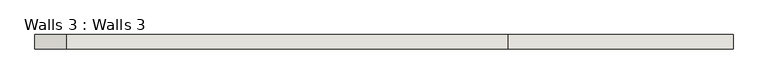
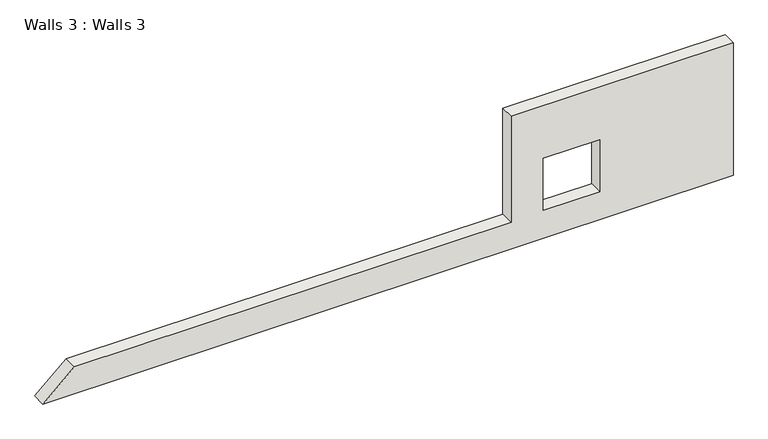
"""IFC4 building model written with IfcOpenShell, lengths in millimetres: wall geometry, Walls 3 : Walls 3."""

from ifc_helpers import new_model, si_unit, point, frame, frame_2d, origin, place, context, project, spatial, polyline, circle_curve, trimmed, segment, composite_curve, outline, extrude, source, transform, mapped, element, save


def walls_3_walls_3_95cfad7e(model_context):
    return source(origin(), model_context, "Body", "SweptSolid", [
        extrude(outline(composite_curve([segment(polyline([(3048.0, -7270.1118051), (3048.0, 7741.1425224), (6096.0, 7741.1425224), (6096.0, 2911.6217382), (3666.8387902, 2911.6217382), (3666.8387902, -6585.3227831)]), True, "CONTINUOUS"), segment(trimmed(circle_curve(frame_2d((-2863.3221432, -1306.0790316)), 8397.2267091), [point((3666.8387902, -6585.3227831))], [point((3048.0, -7270.1118051))], False, "CARTESIAN"), True, "CONTINUOUS")], self_intersect=False), holes=[polyline([(3690.0418748, 3611.9909002), (4887.6780725, 3611.9909002), (4887.6780725, 4841.3147473), (3690.0418748, 4841.3147473), (3690.0418748, 3611.9909002)])]), frame((0.0, -893.9851555, 0.0), z_axis=(0.0, 1.0, 0.0), x_axis=(0.0, 0.0, 1.0)), (0.0, 0.0, 1.0), 304.8),
    ])


if __name__ == "__main__":
    model = new_model("IFC4")
    model_context = context("Model", 3, world=origin())
    ifc_project = project(units=[si_unit("LENGTHUNIT", "METRE", prefix="MILLI")], contexts=[model_context])
    site = spatial("IfcSite", under=ifc_project)
    building = spatial("IfcBuilding", under=site)
    placement = place(None, origin())
    walls_3_walls_3_shape = walls_3_walls_3_95cfad7e(model_context)
    element("IfcWall", 1, ObjectType="Walls 3 : Walls 3", at=placement, inside=building, context=model_context, shape_type="MappedRepresentation", body=[
        mapped(walls_3_walls_3_shape, transform((0.0, 0.0, 0.0), x_axis=(1.0, 0.0, 0.0), y_axis=(0.0, 1.0, 0.0), z_axis=(0.0, 0.0, 1.0))),
    ])
    save(model, "model.ifc")

# Revit data of these elements
# Element 1 (IfcWall, "Walls 3 : Walls 3")
#   Materials on its faces: "Default Wall"
# Materials
#   "Default Wall": colour RGB 80 80 80, transparency 0
